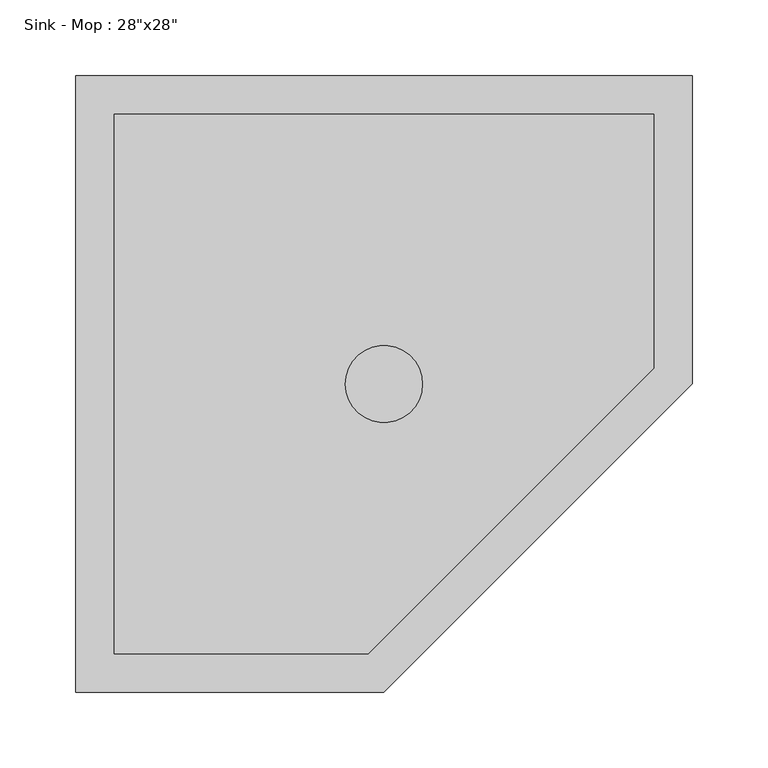
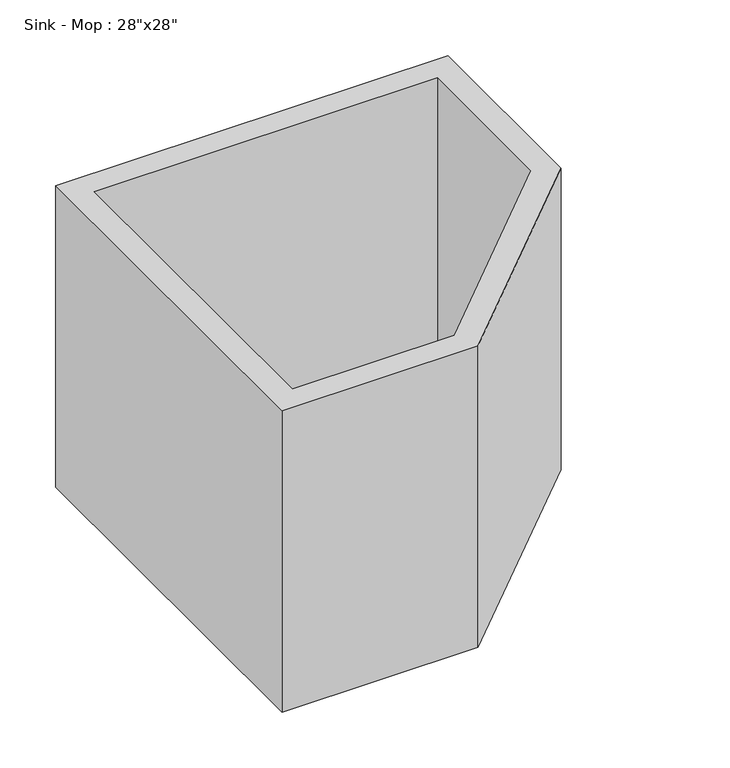
"""IFC4 building model written with IfcOpenShell, lengths in millimetres: flow terminal geometry."""

from ifc_helpers import new_model, si_unit, point, frame, frame_2d, origin, origin_with_axes, place, context, project, spatial, polyline, circle_curve, trimmed, segment, composite_curve, outline, extrude, source, transform, mapped, element, save
from ifc_brep_helpers import plane_surface, revolved_surface, advanced_brep


def flow_terminal_5b58e753(model_context):
    return source(origin(), model_context, "Body", "SolidModel", [
        advanced_brep(
        [(406.4, 0.0, 330.2), (0.0, 0.0, 330.2), (0.0, -406.4, 330.2), (203.2, -406.4, 330.2), (406.4, -203.2, 330.2), (25.4, -25.4, 330.2), (381.0, -25.4, 330.2), (381.0, -192.6789755, 330.2), (192.6789755, -381.0, 330.2), (25.4, -381.0, 330.2), (406.4, 0.0, 0.0), (406.4, -203.2, 0.0), (203.2, -406.4, 0.0), (0.0, -406.4, 0.0), (0.0, 0.0, 0.0), (177.8, -203.2, 0.0), (228.6, -203.2, 0.0), (381.0, -25.4, 25.4), (25.4, -25.4, 25.4), (25.4, -381.0, 25.4), (192.6789755, -381.0, 25.4), (381.0, -192.6789755, 25.4), (228.6, -203.2, 25.4), (177.8, -203.2, 25.4)],
        [
            (0, 1),
            (1, 2),
            (2, 3),
            (3, 4),
            (4, 0),
            (5, 6),
            (6, 7),
            (7, 8),
            (8, 9),
            (9, 5),
            (10, 11),
            (11, 12),
            (12, 13),
            (13, 14),
            (14, 10),
            (15, 16, circle_curve(frame((203.2, -203.2, 0.0), z_axis=(0.0, 0.0, 1.0), x_axis=(1.0, 0.0, 0.0)), 25.4)),
            (16, 15, circle_curve(frame((203.2, -203.2, 0.0), z_axis=(0.0, 0.0, 1.0), x_axis=(1.0, 0.0, 0.0)), 25.4)),
            (0, 10),
            (14, 1),
            (13, 2),
            (12, 3),
            (11, 4),
            (17, 18),
            (18, 19),
            (19, 20),
            (20, 21),
            (21, 17),
            (22, 23, circle_curve(frame((203.2, -203.2, 25.4), z_axis=(0.0, 0.0, -1.0), x_axis=(1.0, 0.0, 0.0)), 25.4)),
            (23, 22, circle_curve(frame((203.2, -203.2, 25.4), z_axis=(0.0, 0.0, -1.0), x_axis=(1.0, 0.0, 0.0)), 25.4)),
            (17, 6),
            (5, 18),
            (9, 19),
            (8, 20),
            (7, 21),
            (22, 16),
            (15, 23),
        ],
        [
            plane_surface(frame((0.0, 0.0, 330.2), z_axis=(0.0, 0.0, 1.0), x_axis=(-1.0, 0.0, 0.0))),
            plane_surface(frame((0.0, 0.0, 0.0), z_axis=(0.0, 0.0, -1.0), x_axis=(1.0, 0.0, 0.0))),
            plane_surface(frame((406.4, 0.0, 330.2), z_axis=(0.0, 1.0, 0.0), x_axis=(0.0, 0.0, -1.0))),
            plane_surface(frame((0.0, 0.0, 330.2), z_axis=(-1.0, 0.0, 0.0), x_axis=(0.0, 0.0, -1.0))),
            plane_surface(frame((0.0, -406.4, 330.2), z_axis=(0.0, -1.0, 0.0), x_axis=(0.0, 0.0, -1.0))),
            plane_surface(frame((203.2, -406.4, 330.2), z_axis=(0.7071067811865448, -0.7071067811865503, 0.0), x_axis=(0.0, 0.0, -1.0))),
            plane_surface(frame((406.4, -203.2, 330.2), z_axis=(1.0, 0.0, 0.0), x_axis=(0.0, 0.0, -1.0))),
            plane_surface(frame((25.4, -25.4, 25.4), z_axis=(0.0, 0.0, 1.0), x_axis=(1.0, 0.0, 0.0))),
            plane_surface(frame((381.0, -25.4, 330.2), z_axis=(0.0, -1.0, 0.0), x_axis=(0.0, 0.0, -1.0))),
            plane_surface(frame((25.4, -25.4, 330.2), z_axis=(1.0, 0.0, 0.0), x_axis=(0.0, 0.0, -1.0))),
            plane_surface(frame((25.4, -381.0, 330.2), z_axis=(0.0, 1.0, 0.0), x_axis=(0.0, 0.0, -1.0))),
            plane_surface(frame((192.6789755, -381.0, 330.2), z_axis=(-0.7071067811865605, 0.7071067811865346, 0.0), x_axis=(0.0, 0.0, -1.0))),
            plane_surface(frame((381.0, -192.6789755, 330.2), z_axis=(-1.0, 0.0, 0.0), x_axis=(0.0, 0.0, -1.0))),
            revolved_surface(polyline([(228.6, -203.2, 25.4), (228.6, -203.2, 0.0)]), (203.2, -203.2, 0.0), (0.0, 0.0, 1.0)),
        ],
        [
            (0, [[1, 2, 3, 4, 5], [6, 7, 8, 9, 10]]),
            (1, [[11, 12, 13, 14, 15], [16, 17]]),
            (2, [[-1, 18, -15, 19]]),
            (3, [[-2, -19, -14, 20]]),
            (4, [[-3, -20, -13, 21]]),
            (5, [[-4, -21, -12, 22]]),
            (6, [[-5, -22, -11, -18]]),
            (7, [[23, 24, 25, 26, 27], [28, 29]]),
            (8, [[-23, 30, -6, 31]]),
            (9, [[-24, -31, -10, 32]]),
            (10, [[-25, -32, -9, 33]]),
            (11, [[-26, -33, -8, 34]]),
            (12, [[-27, -34, -7, -30]]),
            (13, [[35, -16, 36, -28]]),
            (13, [[-35, -29, -36, -17]]),
        ],
    ),
        extrude(outline(composite_curve([segment(trimmed(circle_curve(frame_2d((203.2, -203.2)), 25.4), [point((177.8, -203.2))], [point((228.6, -203.2))], False, "CARTESIAN"), True, "CONTINUOUS"), segment(trimmed(circle_curve(frame_2d((203.2, -203.2)), 25.4), [point((228.6, -203.2))], [point((177.8, -203.2))], False, "CARTESIAN"), True, "CONTINUOUS")], self_intersect=False)), origin_with_axes(), (0.0, 0.0, 1.0), 25.4),
    ])


if __name__ == "__main__":
    model = new_model("IFC4")
    model_context = context("Model", 3, world=origin())
    ifc_project = project(units=[si_unit("LENGTHUNIT", "METRE", prefix="MILLI")], contexts=[model_context])
    site = spatial("IfcSite", under=ifc_project)
    building = spatial("IfcBuilding", under=site)
    placement = place(None, origin())
    flow_terminal_shape = flow_terminal_5b58e753(model_context)
    element("IfcFlowTerminal", 1, ObjectType="Sink - Mop : 28\"x28\"", at=placement, inside=building, context=model_context, shape_type="MappedRepresentation", body=[
        mapped(flow_terminal_shape, transform((0.0, 0.0, 0.0), x_axis=(1.0, 0.0, 0.0), y_axis=(0.0, 1.0, 0.0), z_axis=(0.0, 0.0, 1.0))),
    ])
    save(model, "model.ifc")

# Revit data of these elements
# Type "Sink - Mop : 28\"x28\""
#   WFU = 2
#   Sink Width = 1' - 4"
#   Sink Length = 1' - 4"
#   Sanitary Radius = 1"
#   Sanitary Diameter = 2"
#   Half Sink Width = 0' - 8"
#   Half Sink Length = 0' - 8"
#   Sink Material = none
#   HWFU = 0
#   Default Elevation = 0
#   CWFU = 0
#   Assembly Code = ""
